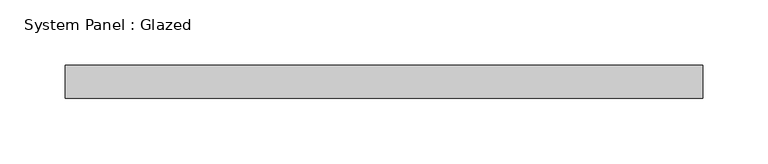
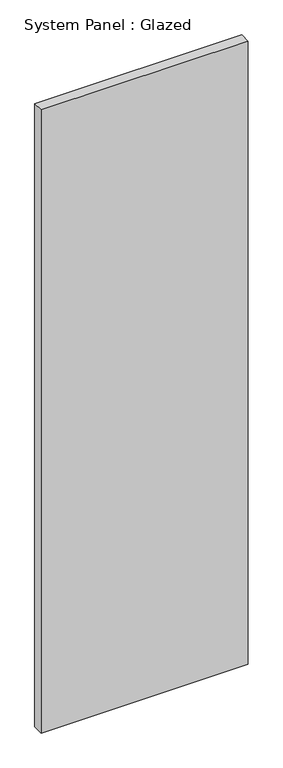
"""IFC4 building model written with IfcOpenShell, lengths in millimetres: plate geometry, System Panel : Glazed."""

from ifc_helpers import new_model, si_unit, origin, origin_with_axes, place, context, project, spatial, polyline, outline, extrude, source, transform, mapped, element, save


def system_panel_glazed_4e9385f6(model_context):
    return source(origin(), model_context, "Body", "SweptSolid", [
        extrude(outline(polyline([(244.475, 19.05), (-244.475, 19.05), (-244.475, 44.45), (244.475, 44.45), (244.475, 19.05)])), origin_with_axes(), (0.0, 0.0, 1.0), 1554.1349385),
    ])


if __name__ == "__main__":
    model = new_model("IFC4")
    model_context = context("Model", 3, world=origin())
    ifc_project = project(units=[si_unit("LENGTHUNIT", "METRE", prefix="MILLI")], contexts=[model_context])
    site = spatial("IfcSite", under=ifc_project)
    building = spatial("IfcBuilding", under=site)
    placement = place(None, origin())
    system_panel_glazed_shape = system_panel_glazed_4e9385f6(model_context)
    element("IfcPlate", 1, ObjectType="System Panel : Glazed", at=placement, inside=building, context=model_context, shape_type="MappedRepresentation", body=[
        mapped(system_panel_glazed_shape, transform((0.0, 0.0, 0.0), x_axis=(1.0, 0.0, 0.0), y_axis=(0.0, 1.0, 0.0), z_axis=(0.0, 0.0, 1.0))),
    ])
    save(model, "model.ifc")

# Revit data of these elements
# Type "System Panel : Glazed"
#   Construction Type Id = "GSP4R"
#   Analytic Construction = "1/8 in Pilkington single glazing"
#   Visual Light Transmittance = 0.9
#   Solar Heat Gain Coefficient = 0.86
#   Heat Transfer Coefficient (U) = 1.18115 BTU/(h·ft²·°F)
#   Define Thermal Properties by = 1
# Element 1 (IfcPlate, "System Panel : Glazed")
#   Materials on its faces: "Glass"
# Materials
#   "Glass": class "Glass", colour RGB 0 128 192, transparency 0.75, Description = "Soda Lime Glass", Cost = 0
